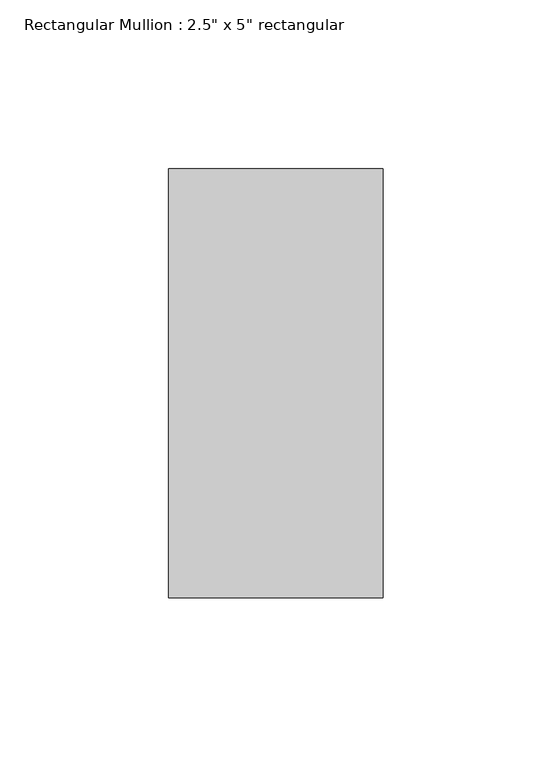
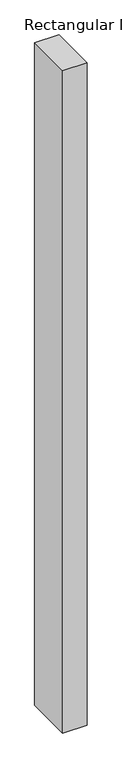
"""IFC4 building model written with IfcOpenShell, lengths in millimetres: member geometry."""

from ifc_helpers import new_model, si_unit, frame, origin, place, context, project, spatial, polyline, outline, extrude, source, transform, mapped, element, save


def member_d60e8053(model_context):
    return source(origin(), model_context, "Body", "SweptSolid", [
        extrude(outline(polyline([(31.75, 63.5), (31.75, -63.5), (-31.75, -63.5), (-31.75, 63.5), (31.75, 63.5)])), frame((0.0, 0.0, -1828.8), z_axis=(0.0, 0.0, 1.0), x_axis=(1.0, 0.0, 0.0)), (0.0, 0.0, 1.0), 1828.8),
    ])


if __name__ == "__main__":
    model = new_model("IFC4")
    model_context = context("Model", 3, world=origin())
    ifc_project = project(units=[si_unit("LENGTHUNIT", "METRE", prefix="MILLI")], contexts=[model_context])
    site = spatial("IfcSite", under=ifc_project)
    building = spatial("IfcBuilding", under=site)
    placement = place(None, origin())
    member_shape = member_d60e8053(model_context)
    element("IfcMember", 1, ObjectType="Rectangular Mullion : 2.5\" x 5\" rectangular", at=placement, inside=building, context=model_context, shape_type="MappedRepresentation", body=[
        mapped(member_shape, transform((0.0, 0.0, 0.0), x_axis=(1.0, 0.0, 0.0), y_axis=(0.0, 1.0, 0.0), z_axis=(0.0, 0.0, 1.0))),
    ])
    save(model, "model.ifc")

# Revit data of these elements
# Type "Rectangular Mullion : 2.5\" x 5\" rectangular"
#   built-in parameter 1007304 = 0.416667 (stored number, unit not read)
#   built-in parameter 1007301 = 0.104167 (stored number, unit not read)
#   built-in parameter 1007300 = 0.104167 (stored number, unit not read)
# Element 1 (IfcMember, "Rectangular Mullion : 2.5\" x 5\" rectangular")
#   Materials on its faces: "Iron, Ductile"
# Materials
#   "Iron, Ductile": class "Metal", colour RGB 0 0 0, transparency 0, Description = "Ductile cast iron", Cost = 0
